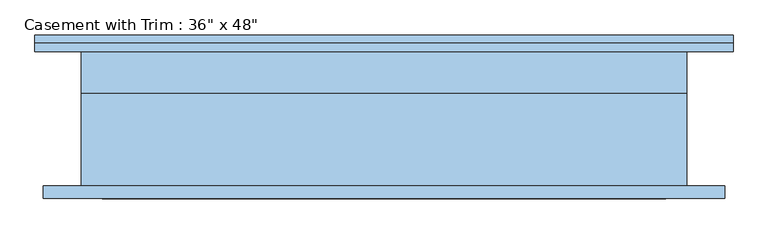
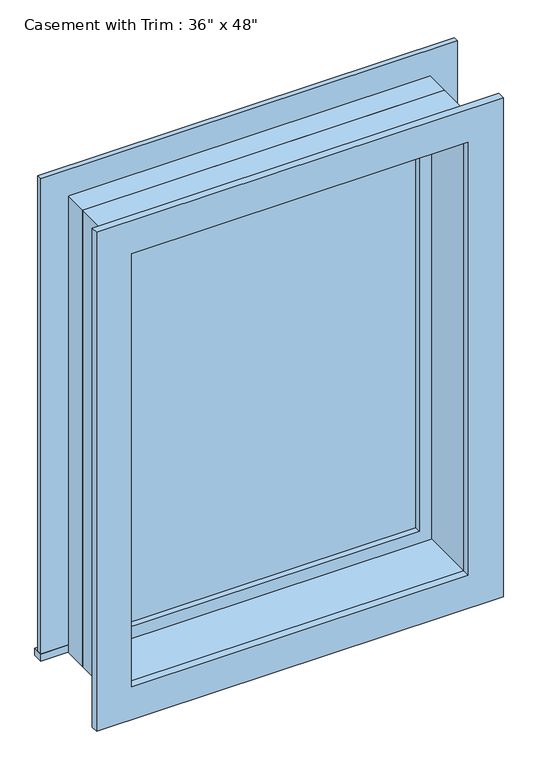
"""IFC4 building model written with IfcOpenShell, lengths in millimetres: window geometry."""

from ifc_helpers import new_model, si_unit, frame, origin, place, context, project, spatial, polyline, outline, extrude, source, transform, mapped, element, save


def window_8a4441b2(model_context):
    return source(origin(), model_context, "Body", "SweptSolid", [
        extrude(outline(polyline([(-527.05, 127.0), (527.05, 127.0), (527.05, 101.6), (-527.05, 101.6), (-527.05, 127.0)])), frame((0.0, 0.0, 914.4), z_axis=(0.0, 0.0, 1.0), x_axis=(1.0, 0.0, 0.0)), (0.0, 0.0, 1.0), 19.05),
        extrude(outline(polyline([(2114.55, -438.15), (2114.55, 438.15), (933.45, 438.15), (933.45, 527.05), (2203.45, 527.05), (2203.45, -527.05), (933.45, -527.05), (933.45, -438.15), (2114.55, -438.15)])), frame((0.0, 101.6, 0.0), z_axis=(0.0, 1.0, 0.0), x_axis=(0.0, 0.0, 1.0)), (0.0, 0.0, 1.0), 12.7),
        extrude(outline(polyline([(2190.75, 514.35), (2190.75, -514.35), (857.25, -514.35), (857.25, 514.35), (2190.75, 514.35)]), holes=[polyline([(2101.85, 425.45), (946.15, 425.45), (946.15, -425.45), (2101.85, -425.45), (2101.85, 425.45)])]), frame((0.0, -120.65, 0.0), z_axis=(0.0, 1.0, 0.0), x_axis=(0.0, 0.0, 1.0)), (0.0, 0.0, 1.0), 19.05),
        extrude(outline(polyline([(393.7, 53.975), (-393.7, 53.975), (-393.7, 66.675), (393.7, 66.675), (393.7, 53.975)])), frame((0.0, 0.0, 977.9), z_axis=(0.0, 0.0, 1.0), x_axis=(1.0, 0.0, 0.0)), (0.0, 0.0, 1.0), 1092.2),
        extrude(outline(polyline([(2114.55, -438.15), (933.45, -438.15), (933.45, 438.15), (2114.55, 438.15), (2114.55, -438.15)]), holes=[polyline([(2070.1, -393.7), (2070.1, 393.7), (977.9, 393.7), (977.9, -393.7), (2070.1, -393.7)])]), frame((0.0, 38.1, 0.0), z_axis=(0.0, 1.0, 0.0), x_axis=(0.0, 0.0, 1.0)), (0.0, 0.0, 1.0), 44.45),
        extrude(outline(polyline([(2133.6, -457.2), (914.4, -457.2), (914.4, 457.2), (2133.6, 457.2), (2133.6, -457.2)]), holes=[polyline([(2101.85, -425.45), (2101.85, 425.45), (946.15, 425.45), (946.15, -425.45), (2101.85, -425.45)])]), frame((0.0, -101.6, 0.0), z_axis=(0.0, 1.0, 0.0), x_axis=(0.0, 0.0, 1.0)), (0.0, 0.0, 1.0), 139.7),
        extrude(outline(polyline([(2133.6, 457.2), (2133.6, -457.2), (914.4, -457.2), (914.4, 457.2), (2133.6, 457.2)]), holes=[polyline([(2114.55, 438.15), (933.45, 438.15), (933.45, -438.15), (2114.55, -438.15), (2114.55, 438.15)])]), frame((0.0, 38.1, 0.0), z_axis=(0.0, 1.0, 0.0), x_axis=(0.0, 0.0, 1.0)), (0.0, 0.0, 1.0), 63.5),
    ])


if __name__ == "__main__":
    model = new_model("IFC4")
    model_context = context("Model", 3, world=origin())
    ifc_project = project(units=[si_unit("LENGTHUNIT", "METRE", prefix="MILLI")], contexts=[model_context])
    site = spatial("IfcSite", under=ifc_project)
    building = spatial("IfcBuilding", under=site)
    placement = place(None, origin())
    window_shape = window_8a4441b2(model_context)
    element("IfcWindow", 1, ObjectType="Casement with Trim : 36\" x 48\"", at=placement, inside=building, context=model_context, shape_type="MappedRepresentation", body=[
        mapped(window_shape, transform((0.0, 0.0, 0.0), x_axis=(1.0, 0.0, 0.0), y_axis=(0.0, 1.0, 0.0), z_axis=(0.0, 0.0, 1.0))),
    ])
    save(model, "model.ifc")

# Revit data of these elements
# Type "Casement with Trim : 36\" x 48\""
#   Type Mark = "29"
#   Construction Type Id = "GSP4R"
#   Assembly Code = "B2020100"
#   Analytic Construction = "1/8 in Pilkington single glazing"
#   Visual Light Transmittance = 0.9
#   Solar Heat Gain Coefficient = 0.78
#   Heat Transfer Coefficient (U) = 0.6496 BTU/(h·ft²·°F)
#   Height = 4' - 0"
#   Default Sill Height = 3' - 0"
#   Trim Projection - Ext. = 0' - 0 1/2"
#   Trim Projection - Int. = 0' - 0 3/4"
#   Trim Width - Exterior = 0' - 3 1/2"
#   Trim Width - Interior = 0' - 3 1/2"
#   Width = 3' - 0"
#   Window Inset = 0' - 0 3/4"
#   Define Thermal Properties by = 1
#   Glass Pane Material = Glass
#   Sash Material = Sash
#   Trim Exterior Material = Trim
#   Trim Interior Material = Trim
#   Wall Closure = (empty or 0)
# Element 1 (IfcWindow, "Casement with Trim : 36\" x 48\"")
#   Materials on its faces: "Sash", "Trim", "Glass"
# Materials
#   "Glass": class "Glass", colour RGB 0 128 192, transparency 0.75, Description = "Soda Lime Glass", Cost = 0
#   "Sash": class "Wood", colour RGB 224 178 126, transparency 0
#   "Trim": class "Wood", colour RGB 224 178 126, transparency 0
